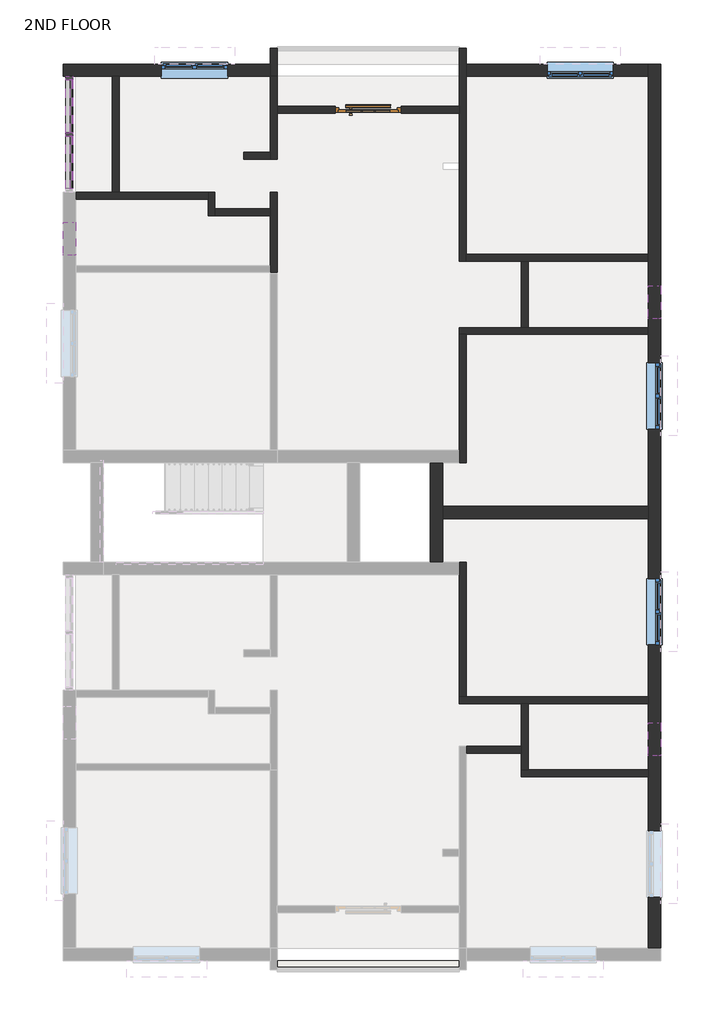
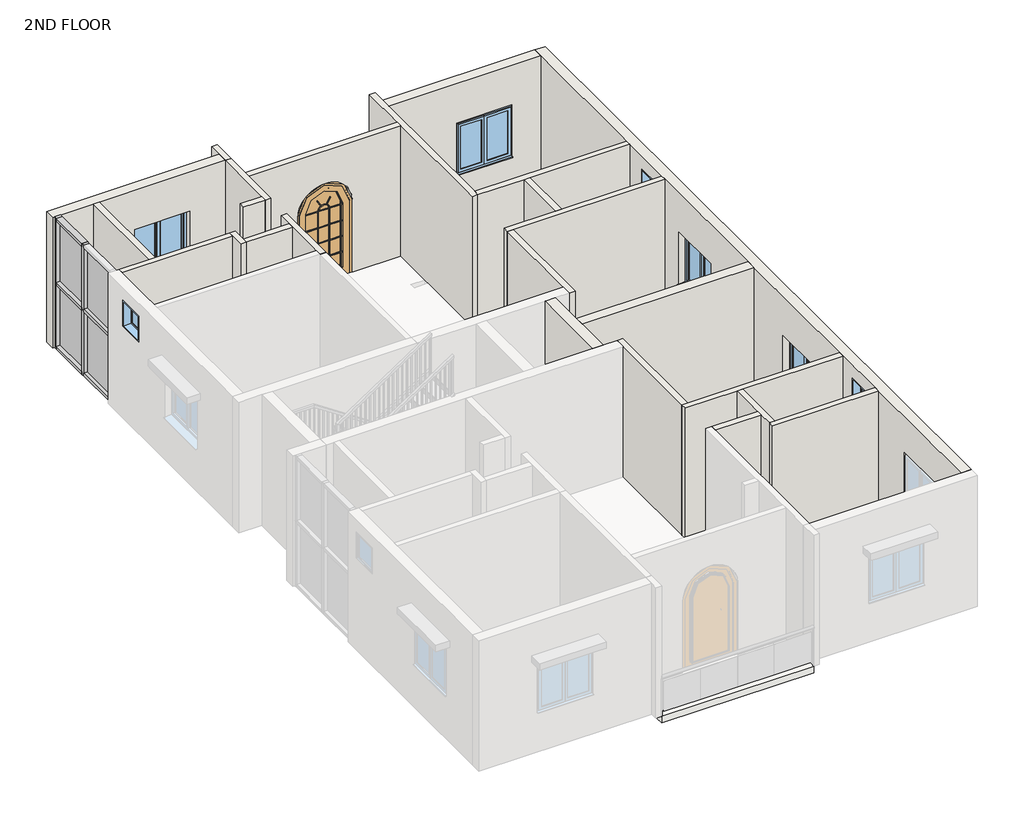
# One storey, part 2 of 4: 24 walls, 9 members, 7 windows, 4 plates, 1 door, 1 slab.
"""IFC4 building model written with IfcOpenShell, lengths in millimetres."""

from ifc_helpers import new_model, si_unit, point, frame, frame_2d, origin, place, context, project, spatial, polyline, circle_curve, trimmed, segment, composite_curve, outline, extrude, faceted_brep, transform, mapped, element, save
from components import door_arched_single_french_glass_wood_exterior_4_x_7_french_5c4dec95, member_801a2072, member_82905deb, member_88aa5c81, member_4491d118, system_panel_glazed_a8655be6, window_80340324, w2_windows_4_x_4_9dec5fc7

model = new_model("IFC4")

# Units and contexts
model_context = context("Model", 3, world=origin())
ifc_project = project(units=[si_unit("LENGTHUNIT", "METRE", prefix="MILLI")], contexts=[model_context])

# Site, building, storey
site = spatial("IfcSite", under=ifc_project)
building = spatial("IfcBuilding", under=site)
storey = spatial("IfcBuildingStorey", under=building, Name="2ND FLOOR", Elevation=9144.0)

# Door
placement = place(None, origin())
door_arched_single_french_glass_wood_exterior_4_x_7_french_shape = door_arched_single_french_glass_wood_exterior_4_x_7_french_5c4dec95(model_context)
element("IfcDoor", 1, ObjectType="Door_Arched_Single_French_Glass_Wood_Exterior : 4' x 7' french door", at=placement, inside=storey, context=model_context, shape_type="MappedRepresentation", body=[
    mapped(door_arched_single_french_glass_wood_exterior_4_x_7_french_shape, transform((-817.6012202, 12433.0309003, 9144.0), x_axis=(1.0, 0.0, 0.0), y_axis=(0.0, 1.0, 0.0), z_axis=(0.0, 0.0, 1.0))),
])

# Members
member_shape = member_801a2072(model_context)
element("IfcMember", 2, ObjectType="Rectangular Mullion : 2.5\" x 5\" rectangular", at=placement, inside=storey, context=model_context, shape_type="MappedRepresentation", body=[
    mapped(member_shape, transform((-6318.2887202, 12007.5809003, 12192.0), x_axis=(0.0, 0.0, 1.0), y_axis=(-1.0, 0.0, 0.0), z_axis=(0.0, -1.0, 0.0))),
])
element("IfcMember", 3, ObjectType="Rectangular Mullion : 2.5\" x 5\" rectangular", at=placement, inside=storey, context=model_context, shape_type="MappedRepresentation", body=[
    mapped(member_shape, transform((-6318.2887202, 12979.1309003, 9144.0), x_axis=(0.0, 0.0, -1.0), y_axis=(-1.0, 0.0, 0.0), z_axis=(0.0, 1.0, 0.0))),
])
element("IfcMember", 4, ObjectType="Rectangular Mullion : 2.5\" x 5\" rectangular", at=placement, inside=storey, context=model_context, shape_type="MappedRepresentation", body=[
    mapped(member_shape, transform((-6318.2887202, 11944.0809003, 9144.0), x_axis=(0.0, 0.0, -1.0), y_axis=(-1.0, 0.0, 0.0), z_axis=(0.0, 1.0, 0.0))),
])
member_2_shape = member_82905deb(model_context)
element("IfcMember", 5, ObjectType="Rectangular Mullion : 2.5\" x 5\" rectangular", at=placement, inside=storey, context=model_context, shape_type="MappedRepresentation", body=[
    mapped(member_2_shape, transform((-6318.2887202, 11975.8309003, 9144.0), x_axis=(0.0, -1.0, 0.0), y_axis=(-1.0, 0.0, 0.0), z_axis=(0.0, 0.0, -1.0))),
])
member_3_shape = member_88aa5c81(model_context)
element("IfcMember", 6, ObjectType="Rectangular Mullion : 2.5\" x 5\" rectangular", at=placement, inside=storey, context=model_context, shape_type="MappedRepresentation", body=[
    mapped(member_3_shape, transform((-6318.2887202, 12007.5809003, 10668.0), x_axis=(0.0, 0.0, 1.0), y_axis=(-1.0, 0.0, 0.0), z_axis=(0.0, -1.0, 0.0))),
])
element("IfcMember", 7, ObjectType="Rectangular Mullion : 2.5\" x 5\" rectangular", at=placement, inside=storey, context=model_context, shape_type="MappedRepresentation", body=[
    mapped(member_3_shape, transform((-6318.2887202, 10972.5309003, 10668.0), x_axis=(0.0, 0.0, 1.0), y_axis=(-1.0, 0.0, 0.0), z_axis=(0.0, -1.0, 0.0))),
])
element("IfcMember", 8, ObjectType="Rectangular Mullion : 2.5\" x 5\" rectangular", at=placement, inside=storey, context=model_context, shape_type="MappedRepresentation", body=[
    mapped(member_2_shape, transform((-6318.2887202, 11975.8309003, 10668.0), x_axis=(0.0, -1.0, 0.0), y_axis=(-1.0, 0.0, 0.0), z_axis=(0.0, 0.0, -1.0))),
])
member_4_shape = member_4491d118(model_context)
element("IfcMember", 9, ObjectType="Rectangular Mullion : 2.5\" x 5\" rectangular", at=placement, inside=storey, context=model_context, shape_type="MappedRepresentation", body=[
    mapped(member_4_shape, transform((-6318.2887202, 13042.6309003, 12192.0), x_axis=(0.0, 1.0, 0.0), y_axis=(-1.0, 0.0, 0.0), z_axis=(0.0, 0.0, 1.0))),
])
element("IfcMember", 10, ObjectType="Rectangular Mullion : 2.5\" x 5\" rectangular", at=placement, inside=storey, context=model_context, shape_type="MappedRepresentation", body=[
    mapped(member_4_shape, transform((-6318.2887202, 13042.6309003, 10668.0), x_axis=(0.0, 1.0, 0.0), y_axis=(-1.0, 0.0, 0.0), z_axis=(0.0, 0.0, 1.0))),
])

# Plates
system_panel_glazed_shape = system_panel_glazed_a8655be6(model_context)
element("IfcPlate", 11, ObjectType="System Panel : Glazed", at=placement, inside=storey, context=model_context, shape_type="MappedRepresentation", body=[
    mapped(system_panel_glazed_shape, transform((-6318.2887202, 12493.3559003, 9207.5), x_axis=(0.0, -1.0, 0.0), y_axis=(1.0, 0.0, 0.0), z_axis=(0.0, 0.0, 1.0))),
])
element("IfcPlate", 12, ObjectType="System Panel : Glazed", at=placement, inside=storey, context=model_context, shape_type="MappedRepresentation", body=[
    mapped(system_panel_glazed_shape, transform((-6318.2887202, 11458.3059003, 9207.5), x_axis=(0.0, -1.0, 0.0), y_axis=(1.0, 0.0, 0.0), z_axis=(0.0, 0.0, 1.0))),
])
element("IfcPlate", 13, ObjectType="System Panel : Glazed", at=placement, inside=storey, context=model_context, shape_type="MappedRepresentation", body=[
    mapped(system_panel_glazed_shape, transform((-6318.2887202, 12493.3559003, 10699.75), x_axis=(0.0, -1.0, 0.0), y_axis=(1.0, 0.0, 0.0), z_axis=(0.0, 0.0, 1.0))),
])
element("IfcPlate", 14, ObjectType="System Panel : Glazed", at=placement, inside=storey, context=model_context, shape_type="MappedRepresentation", body=[
    mapped(system_panel_glazed_shape, transform((-6318.2887202, 11458.3059003, 10699.75), x_axis=(0.0, -1.0, 0.0), y_axis=(1.0, 0.0, 0.0), z_axis=(0.0, 0.0, 1.0))),
])

# Slab
element("IfcSlab", 15, ObjectType="bathroom tiles", at=placement, inside=storey, context=model_context, shape_type="SweptSolid", body=[
    extrude(outline(polyline([(858.7987798, -3238.7690997), (858.7987798, -3403.8690997), (-2494.0012202, -3403.8690997), (-2494.0012202, -3238.7690997), (858.7987798, -3238.7690997)])), frame((0.0, 0.0, 8991.6), z_axis=(0.0, 0.0, 1.0), x_axis=(1.0, 0.0, 0.0)), (0.0, 0.0, 1.0), 152.4),
])

# Walls
element("IfcWall", 16, ObjectType="OUTER WALL 9\"", at=placement, inside=storey, context=model_context, shape_type="Brep", body=[
    faceted_brep([(4567.1987798, -3010.1690997, 9144.0), (4567.1987798, 13271.2309003, 9144.0), (4567.1987798, 13271.2309003, 12192.0), (4567.1987798, -3010.1690997, 12192.0), (4567.1987798, -844.8190997, 11363.2), (4567.1987798, -844.8190997, 10144.0), (4567.1987798, -2064.0190997, 10144.0), (4567.1987798, -2064.0190997, 11363.2), (4567.1987798, 2577.8309003, 10058.4), (4567.1987798, 2577.8309003, 11277.6), (4567.1987798, 3797.0309003, 11277.6), (4567.1987798, 3797.0309003, 10058.4), (4567.1987798, 6552.9309003, 10058.4), (4567.1987798, 6552.9309003, 11277.6), (4567.1987798, 7772.1309003, 11277.6), (4567.1987798, 7772.1309003, 10058.4), (4567.1987798, 539.4809003, 11277.6), (4567.1987798, 539.4809003, 11887.2), (4567.1987798, 1149.0809003, 11887.2), (4567.1987798, 1149.0809003, 11277.6), (4567.1987798, 8584.9309003, 11277.6), (4567.1987798, 8584.9309003, 11887.2), (4567.1987798, 9194.5309003, 11887.2), (4567.1987798, 9194.5309003, 11277.6), (4338.5987798, 13271.2309003, 9144.0), (4338.5987798, 13042.6309003, 9144.0), (4338.5987798, 9766.0309003, 9144.0), (4338.5987798, 9639.0309003, 9144.0), (4338.5987798, 8419.8309003, 9144.0), (4338.5987798, 8292.8309003, 9144.0), (4338.5987798, 5130.5309003, 9144.0), (4338.5987798, 4901.9309003, 9144.0), (4338.5987798, 1625.3309003, 9144.0), (4338.5987798, 1498.3309003, 9144.0), (4338.5987798, 279.1309003, 9144.0), (4338.5987798, 152.1309003, 9144.0), (4338.5987798, -3010.1690997, 9144.0), (4338.5987798, -3010.1690997, 12192.0), (4338.5987798, 152.1309003, 12192.0), (4338.5987798, 279.1309003, 12192.0), (4338.5987798, 1498.3309003, 12192.0), (4338.5987798, 1625.3309003, 12192.0), (4338.5987798, 4901.9309003, 12192.0), (4338.5987798, 5130.5309003, 12192.0), (4338.5987798, 8292.8309003, 12192.0), (4338.5987798, 8419.8309003, 12192.0), (4338.5987798, 9639.0309003, 12192.0), (4338.5987798, 9766.0309003, 12192.0), (4338.5987798, 13042.6309003, 12192.0), (4338.5987798, 13271.2309003, 12192.0), (4338.5987798, -844.8190997, 10144.0), (4338.5987798, -844.8190997, 11363.2), (4338.5987798, -2064.0190997, 11363.2), (4338.5987798, -2064.0190997, 10144.0), (4338.5987798, 2577.8309003, 11277.6), (4338.5987798, 2577.8309003, 10058.4), (4338.5987798, 3797.0309003, 10058.4), (4338.5987798, 3797.0309003, 11277.6), (4338.5987798, 6552.9309003, 11277.6), (4338.5987798, 6552.9309003, 10058.4), (4338.5987798, 7772.1309003, 10058.4), (4338.5987798, 7772.1309003, 11277.6), (4338.5987798, 539.4809003, 11887.2), (4338.5987798, 539.4809003, 11277.6), (4338.5987798, 1149.0809003, 11277.6), (4338.5987798, 1149.0809003, 11887.2), (4338.5987798, 8584.9309003, 11887.2), (4338.5987798, 8584.9309003, 11277.6), (4338.5987798, 9194.5309003, 11277.6), (4338.5987798, 9194.5309003, 11887.2)], [[[0, 1, 2, 3], [4, 5, 6, 7], [8, 9, 10, 11], [12, 13, 14, 15], [16, 17, 18, 19], [20, 21, 22, 23]], [[24, 25, 26, 27, 28, 29, 30, 31, 32, 33, 34, 35, 36, 37, 38, 39, 40, 41, 42, 43, 44, 45, 46, 47, 48, 49], [50, 51, 52, 53], [54, 55, 56, 57], [58, 59, 60, 61], [62, 63, 64, 65], [66, 67, 68, 69]], [[1, 0, 36, 35, 34, 33, 32, 31, 30, 29, 28, 27, 26, 25, 24]], [[3, 2, 49, 48, 47, 46, 45, 44, 43, 42, 41, 40, 39, 38, 37]], [[0, 3, 37, 36]], [[2, 1, 24, 49]], [[51, 50, 5, 4]], [[52, 51, 4, 7]], [[53, 52, 7, 6]], [[50, 53, 6, 5]], [[9, 8, 55, 54]], [[10, 9, 54, 57]], [[11, 10, 57, 56]], [[8, 11, 56, 55]], [[13, 12, 59, 58]], [[14, 13, 58, 61]], [[15, 14, 61, 60]], [[12, 15, 60, 59]], [[63, 62, 17, 16]], [[64, 63, 16, 19]], [[65, 64, 19, 18]], [[62, 65, 18, 17]], [[67, 66, 21, 20]], [[68, 67, 20, 23]], [[69, 68, 23, 22]], [[66, 69, 22, 21]]]),
])
element("IfcWall", 17, ObjectType="OUTER WALL 9\"", at=placement, inside=storey, context=model_context, shape_type="SweptSolid", body=[
    extrude(outline(polyline([(9144.0, 4338.5987798), (12192.0, 4338.5987798), (12192.0, 985.7987798), (9144.0, 985.7987798), (9144.0, 4338.5987798)]), holes=[polyline([(10058.4, 2479.7847416), (11277.6, 2479.7847416), (11277.6, 3698.9847416), (10058.4, 3698.9847416), (10058.4, 2479.7847416)])]), frame((0.0, 13042.6309003, 0.0), z_axis=(0.0, 1.0, 0.0), x_axis=(0.0, 0.0, 1.0)), (0.0, 0.0, 1.0), 228.6),
])
element("IfcWall", 18, ObjectType="OUTER WALL 9\"", at=placement, inside=storey, context=model_context, shape_type="Brep", body=[
    faceted_brep([(-2621.0012202, 13271.2309003, 9144.0), (-6432.5887202, 13271.2309003, 9144.0), (-6432.5887202, 13271.2309003, 12192.0), (-2621.0012202, 13271.2309003, 12192.0), (-3402.0512202, 13271.2309003, 10058.4), (-3402.0512202, 13271.2309003, 11277.6), (-4621.2512202, 13271.2309003, 11277.6), (-4621.2512202, 13271.2309003, 10058.4), (-2621.0012202, 13042.6309003, 9144.0), (-2621.0012202, 13042.6309003, 12192.0), (-5402.3012202, 13042.6309003, 12192.0), (-5529.3012202, 13042.6309003, 12192.0), (-6432.5887202, 13042.6309003, 12192.0), (-6432.5887202, 13042.6309003, 9144.0), (-5529.3012202, 13042.6309003, 9144.0), (-5402.3012202, 13042.6309003, 9144.0), (-3402.0512202, 13042.6309003, 10058.4), (-4621.2512202, 13042.6309003, 10058.4), (-4621.2512202, 13042.6309003, 11277.6), (-3402.0512202, 13042.6309003, 11277.6)], [[[0, 1, 2, 3], [4, 5, 6, 7]], [[8, 9, 10, 11, 12, 13, 14, 15], [16, 17, 18, 19]], [[1, 0, 8, 15, 14, 13]], [[3, 2, 12, 11, 10, 9]], [[2, 1, 13, 12]], [[5, 4, 16, 19]], [[6, 5, 19, 18]], [[7, 6, 18, 17]], [[4, 7, 17, 16]], [[0, 3, 9, 8]]]),
])
element("IfcWall", 19, ObjectType="OUTER WALL 9\"", at=placement, inside=storey, context=model_context, shape_type="Brep", body=[
    faceted_brep([(553.9987798, 4101.8309003, 9144.0), (553.9987798, 4901.9309003, 9144.0), (553.9987798, 5130.5309003, 9144.0), (553.9987798, 5930.6309003, 9144.0), (553.9987798, 5930.6309003, 12192.0), (553.9987798, 5130.5309003, 12192.0), (553.9987798, 4901.9309003, 12192.0), (553.9987798, 4101.8309003, 12192.0), (325.3987798, 4101.8309003, 9144.0), (325.3987798, 4101.8309003, 12192.0), (325.3987798, 5930.6309003, 12192.0), (325.3987798, 5930.6309003, 9144.0)], [[[0, 1, 2, 3, 4, 5, 6, 7]], [[8, 9, 10, 11]], [[3, 2, 1, 0, 8, 11]], [[7, 6, 5, 4, 10, 9]], [[0, 7, 9, 8]], [[4, 3, 11, 10]]]),
])
element("IfcWall", 20, ObjectType="OUTER WALL 9\"", at=placement, inside=storey, context=model_context, shape_type="SweptSolid", body=[
    extrude(outline(polyline([(4338.5987798, 4901.9309003), (553.9987798, 4901.9309003), (553.9987798, 5130.5309003), (4338.5987798, 5130.5309003), (4338.5987798, 4901.9309003)])), frame((0.0, 0.0, 9144.0), z_axis=(0.0, 0.0, 1.0), x_axis=(1.0, 0.0, 0.0)), (0.0, 0.0, 1.0), 3048.0),
])
element("IfcWall", 21, ObjectType="inner wall 5\"", at=placement, inside=storey, context=model_context, shape_type="SweptSolid", body=[
    extrude(outline(polyline([(-5529.3012202, 10909.0309003), (-5529.3012202, 13042.6309003), (-5402.3012202, 13042.6309003), (-5402.3012202, 10909.0309003), (-5529.3012202, 10909.0309003)])), frame((0.0, 0.0, 9144.0), z_axis=(0.0, 0.0, 1.0), x_axis=(1.0, 0.0, 0.0)), (0.0, 0.0, 1.0), 3048.0),
])
element("IfcWall", 22, ObjectType="inner wall 5\"", at=placement, inside=storey, context=model_context, shape_type="Brep", body=[
    faceted_brep([(-2621.0012202, 13042.6309003, 9144.0), (-2621.0012202, 11645.6309003, 9144.0), (-2621.0012202, 11518.6309003, 9144.0), (-2621.0012202, 11518.6309003, 12192.0), (-2621.0012202, 11645.6309003, 12192.0), (-2621.0012202, 13042.6309003, 12192.0), (-2494.0012202, 13042.6309003, 9144.0), (-2494.0012202, 13042.6309003, 12192.0), (-2494.0012202, 12496.5309003, 12192.0), (-2494.0012202, 12369.5309003, 12192.0), (-2494.0012202, 11518.6309003, 12192.0), (-2494.0012202, 11518.6309003, 9144.0), (-2494.0012202, 12369.5309003, 9144.0), (-2494.0012202, 12496.5309003, 9144.0)], [[[0, 1, 2, 3, 4, 5]], [[6, 7, 8, 9, 10, 11, 12, 13]], [[2, 1, 0, 6, 13, 12, 11]], [[5, 4, 3, 10, 9, 8, 7]], [[3, 2, 11, 10]], [[0, 5, 7, 6]]]),
])
element("IfcWall", 23, ObjectType="inner wall 5\"", at=placement, inside=storey, context=model_context, shape_type="SweptSolid", body=[
    extrude(outline(polyline([(-3103.6012202, 11645.6309003), (-2621.0012202, 11645.6309003), (-2621.0012202, 11518.6309003), (-3103.6012202, 11518.6309003), (-3103.6012202, 11645.6309003)])), frame((0.0, 0.0, 9144.0), z_axis=(0.0, 0.0, 1.0), x_axis=(1.0, 0.0, 0.0)), (0.0, 0.0, 1.0), 3048.0),
])
element("IfcWall", 24, ObjectType="inner wall 5\"", at=placement, inside=storey, context=model_context, shape_type="Brep", body=[
    faceted_brep([(-6202.4012202, 10782.0309003, 9144.0), (-3764.0012202, 10782.0309003, 9144.0), (-3764.0012202, 10782.0309003, 12192.0), (-6202.4012202, 10782.0309003, 12192.0), (-6202.4012202, 10909.0309003, 9144.0), (-6202.4012202, 10909.0309003, 12192.0), (-5529.3012202, 10909.0309003, 12192.0), (-5402.3012202, 10909.0309003, 12192.0), (-3764.0012202, 10909.0309003, 12192.0), (-3764.0012202, 10909.0309003, 9144.0), (-5402.3012202, 10909.0309003, 9144.0), (-5529.3012202, 10909.0309003, 9144.0)], [[[0, 1, 2, 3]], [[4, 5, 6, 7, 8, 9, 10, 11]], [[1, 0, 4, 11, 10, 9]], [[3, 2, 8, 7, 6, 5]], [[0, 3, 5, 4]], [[2, 1, 9, 8]]]),
])
element("IfcWall", 25, ObjectType="inner wall 5\"", at=placement, inside=storey, context=model_context, shape_type="Brep", body=[
    faceted_brep([(-3764.0012202, 10909.0309003, 9144.0), (-3764.0012202, 10782.0309003, 9144.0), (-3764.0012202, 10477.2309003, 9144.0), (-3764.0012202, 10477.2309003, 12192.0), (-3764.0012202, 10782.0309003, 12192.0), (-3764.0012202, 10909.0309003, 12192.0), (-3637.0012202, 10909.0309003, 9144.0), (-3637.0012202, 10909.0309003, 12192.0), (-3637.0012202, 10604.2309003, 12192.0), (-3637.0012202, 10477.2309003, 12192.0), (-3637.0012202, 10477.2309003, 9144.0), (-3637.0012202, 10604.2309003, 9144.0)], [[[0, 1, 2, 3, 4, 5]], [[6, 7, 8, 9, 10, 11]], [[2, 1, 0, 6, 11, 10]], [[5, 4, 3, 9, 8, 7]], [[0, 5, 7, 6]], [[3, 2, 10, 9]]]),
])
element("IfcWall", 26, ObjectType="inner wall 5\"", at=placement, inside=storey, context=model_context, shape_type="SweptSolid", body=[
    extrude(outline(polyline([(-2621.0012202, 10477.2309003), (-3637.0012202, 10477.2309003), (-3637.0012202, 10604.2309003), (-2621.0012202, 10604.2309003), (-2621.0012202, 10477.2309003)])), frame((0.0, 0.0, 9144.0), z_axis=(0.0, 0.0, 1.0), x_axis=(1.0, 0.0, 0.0)), (0.0, 0.0, 1.0), 3048.0),
])
element("IfcWall", 27, ObjectType="inner wall 5\"", at=placement, inside=storey, context=model_context, shape_type="Brep", body=[
    faceted_brep([(-2621.0012202, 10909.0309003, 9144.0), (-2621.0012202, 10604.2309003, 9144.0), (-2621.0012202, 10477.2309003, 9144.0), (-2621.0012202, 9562.8309003, 9144.0), (-2621.0012202, 9435.8309003, 9144.0), (-2621.0012202, 9435.8309003, 12192.0), (-2621.0012202, 9562.8309003, 12192.0), (-2621.0012202, 10477.2309003, 12192.0), (-2621.0012202, 10604.2309003, 12192.0), (-2621.0012202, 10909.0309003, 12192.0), (-2494.0012202, 10909.0309003, 9144.0), (-2494.0012202, 10909.0309003, 12192.0), (-2494.0012202, 9435.8309003, 12192.0), (-2494.0012202, 9435.8309003, 9144.0)], [[[0, 1, 2, 3, 4, 5, 6, 7, 8, 9]], [[10, 11, 12, 13]], [[4, 3, 2, 1, 0, 10, 13]], [[9, 8, 7, 6, 5, 12, 11]], [[0, 9, 11, 10]], [[5, 4, 13, 12]]]),
])
element("IfcWall", 28, ObjectType="inner wall 5\"", at=placement, inside=storey, context=model_context, shape_type="SweptSolid", body=[
    extrude(outline(polyline([(2001.7987798, 583.9309003), (985.7987798, 583.9309003), (985.7987798, 710.9309003), (2001.7987798, 710.9309003), (2001.7987798, 583.9309003)])), frame((0.0, 0.0, 9144.0), z_axis=(0.0, 0.0, 1.0), x_axis=(1.0, 0.0, 0.0)), (0.0, 0.0, 1.0), 3048.0),
])
element("IfcWall", 29, ObjectType="inner wall 5\"", at=placement, inside=storey, context=model_context, shape_type="Brep", body=[
    faceted_brep([(4338.5987798, 1625.3309003, 9144.0), (985.7987798, 1625.3309003, 9144.0), (858.7987798, 1625.3309003, 9144.0), (858.7987798, 1625.3309003, 12192.0), (985.7987798, 1625.3309003, 12192.0), (4338.5987798, 1625.3309003, 12192.0), (4338.5987798, 1498.3309003, 9144.0), (4338.5987798, 1498.3309003, 12192.0), (2128.7987798, 1498.3309003, 12192.0), (2001.7987798, 1498.3309003, 12192.0), (858.7987798, 1498.3309003, 12192.0), (858.7987798, 1498.3309003, 9144.0), (2001.7987798, 1498.3309003, 9144.0), (2128.7987798, 1498.3309003, 9144.0)], [[[0, 1, 2, 3, 4, 5]], [[6, 7, 8, 9, 10, 11, 12, 13]], [[2, 1, 0, 6, 13, 12, 11]], [[5, 4, 3, 10, 9, 8, 7]], [[3, 2, 11, 10]], [[0, 5, 7, 6]]]),
])
element("IfcWall", 30, ObjectType="inner wall 5\"", at=placement, inside=storey, context=model_context, shape_type="Brep", body=[
    faceted_brep([(985.7987798, 1625.3309003, 9144.0), (985.7987798, 4101.8309003, 9144.0), (985.7987798, 4101.8309003, 12192.0), (985.7987798, 1625.3309003, 12192.0), (858.7987798, 1625.3309003, 9144.0), (858.7987798, 1625.3309003, 12192.0), (858.7987798, 3873.2309003, 12192.0), (858.7987798, 4101.8309003, 12192.0), (858.7987798, 4101.8309003, 9144.0), (858.7987798, 3873.2309003, 9144.0)], [[[0, 1, 2, 3]], [[4, 5, 6, 7, 8, 9]], [[1, 0, 4, 9, 8]], [[3, 2, 7, 6, 5]], [[0, 3, 5, 4]], [[2, 1, 8, 7]]]),
])
element("IfcWall", 31, ObjectType="inner wall 5\"", at=placement, inside=storey, context=model_context, shape_type="Brep", body=[
    faceted_brep([(4338.5987798, 279.1309003, 9144.0), (2128.7987798, 279.1309003, 9144.0), (2001.7987798, 279.1309003, 9144.0), (2001.7987798, 279.1309003, 12192.0), (2128.7987798, 279.1309003, 12192.0), (4338.5987798, 279.1309003, 12192.0), (4338.5987798, 152.1309003, 9144.0), (4338.5987798, 152.1309003, 12192.0), (2001.7987798, 152.1309003, 12192.0), (2001.7987798, 152.1309003, 9144.0)], [[[0, 1, 2, 3, 4, 5]], [[6, 7, 8, 9]], [[2, 1, 0, 6, 9]], [[5, 4, 3, 8, 7]], [[0, 5, 7, 6]], [[3, 2, 9, 8]]]),
])
element("IfcWall", 32, ObjectType="inner wall 5\"", at=placement, inside=storey, context=model_context, shape_type="Brep", body=[
    faceted_brep([(2128.7987798, 279.1309003, 9144.0), (2128.7987798, 1498.3309003, 9144.0), (2128.7987798, 1498.3309003, 12192.0), (2128.7987798, 279.1309003, 12192.0), (2001.7987798, 279.1309003, 9144.0), (2001.7987798, 279.1309003, 12192.0), (2001.7987798, 583.9309003, 12192.0), (2001.7987798, 710.9309003, 12192.0), (2001.7987798, 1498.3309003, 12192.0), (2001.7987798, 1498.3309003, 9144.0), (2001.7987798, 710.9309003, 9144.0), (2001.7987798, 583.9309003, 9144.0)], [[[0, 1, 2, 3]], [[4, 5, 6, 7, 8, 9, 10, 11]], [[1, 0, 4, 11, 10, 9]], [[3, 2, 8, 7, 6, 5]], [[0, 3, 5, 4]], [[2, 1, 9, 8]]]),
])
element("IfcWall", 33, ObjectType="inner wall 5\"", at=placement, inside=storey, context=model_context, shape_type="SweptSolid", body=[
    extrude(outline(composite_curve([segment(polyline([(10822.6, -208.0012202), (9144.0, -208.0012202), (9144.0, 858.7987798), (12192.0, 858.7987798), (12192.0, -2494.0012202), (9144.0, -2494.0012202), (9144.0, -1427.2012202), (10822.6, -1427.2012202)]), True, "CONTINUOUS"), segment(trimmed(circle_curve(frame_2d((10822.6, -817.6012202)), 609.6), [point((10822.6, -1427.2012202))], [point((10822.6, -208.0012202))], True, "CARTESIAN"), True, "CONTINUOUS")], self_intersect=False)), frame((0.0, 12369.5309003, 0.0), z_axis=(0.0, 1.0, 0.0), x_axis=(0.0, 0.0, 1.0)), (0.0, 0.0, 1.0), 127.0),
])
element("IfcWall", 34, ObjectType="inner wall 5\"", at=placement, inside=storey, context=model_context, shape_type="Brep", body=[
    faceted_brep([(858.7987798, 13563.3309003, 9144.0), (858.7987798, 12496.5309003, 9144.0), (858.7987798, 12369.5309003, 9144.0), (858.7987798, 9639.0309003, 9144.0), (858.7987798, 9639.0309003, 12192.0), (858.7987798, 12369.5309003, 12192.0), (858.7987798, 12496.5309003, 12192.0), (858.7987798, 13563.3309003, 12192.0), (985.7987798, 13563.3309003, 9144.0), (985.7987798, 13563.3309003, 12192.0), (985.7987798, 13271.2309003, 12192.0), (985.7987798, 13042.6309003, 12192.0), (985.7987798, 9766.0309003, 12192.0), (985.7987798, 9639.0309003, 12192.0), (985.7987798, 9639.0309003, 9144.0), (985.7987798, 9766.0309003, 9144.0), (985.7987798, 13042.6309003, 9144.0), (985.7987798, 13271.2309003, 9144.0)], [[[0, 1, 2, 3, 4, 5, 6, 7]], [[8, 9, 10, 11, 12, 13, 14, 15, 16, 17]], [[3, 2, 1, 0, 8, 17, 16, 15, 14]], [[7, 6, 5, 4, 13, 12, 11, 10, 9]], [[0, 7, 9, 8]], [[4, 3, 14, 13]]]),
])
element("IfcWall", 35, ObjectType="inner wall 5\"", at=placement, inside=storey, context=model_context, shape_type="Brep", body=[
    faceted_brep([(4338.5987798, 9766.0309003, 9144.0), (985.7987798, 9766.0309003, 9144.0), (985.7987798, 9766.0309003, 12192.0), (4338.5987798, 9766.0309003, 12192.0), (4338.5987798, 9639.0309003, 9144.0), (4338.5987798, 9639.0309003, 12192.0), (2128.7987798, 9639.0309003, 12192.0), (2001.7987798, 9639.0309003, 12192.0), (985.7987798, 9639.0309003, 12192.0), (985.7987798, 9639.0309003, 9144.0), (2001.7987798, 9639.0309003, 9144.0), (2128.7987798, 9639.0309003, 9144.0)], [[[0, 1, 2, 3]], [[4, 5, 6, 7, 8, 9, 10, 11]], [[1, 0, 4, 11, 10, 9]], [[3, 2, 8, 7, 6, 5]], [[0, 3, 5, 4]], [[2, 1, 9, 8]]]),
])
element("IfcWall", 36, ObjectType="inner wall 5\"", at=placement, inside=storey, context=model_context, shape_type="Brep", body=[
    faceted_brep([(4338.5987798, 8419.8309003, 9144.0), (2128.7987798, 8419.8309003, 9144.0), (2001.7987798, 8419.8309003, 9144.0), (858.7987798, 8419.8309003, 9144.0), (858.7987798, 8419.8309003, 12192.0), (2001.7987798, 8419.8309003, 12192.0), (2128.7987798, 8419.8309003, 12192.0), (4338.5987798, 8419.8309003, 12192.0), (4338.5987798, 8292.8309003, 9144.0), (4338.5987798, 8292.8309003, 12192.0), (985.7987798, 8292.8309003, 12192.0), (858.7987798, 8292.8309003, 12192.0), (858.7987798, 8292.8309003, 9144.0), (985.7987798, 8292.8309003, 9144.0)], [[[0, 1, 2, 3, 4, 5, 6, 7]], [[8, 9, 10, 11, 12, 13]], [[3, 2, 1, 0, 8, 13, 12]], [[7, 6, 5, 4, 11, 10, 9]], [[0, 7, 9, 8]], [[4, 3, 12, 11]]]),
])
element("IfcWall", 37, ObjectType="inner wall 5\"", at=placement, inside=storey, context=model_context, shape_type="SweptSolid", body=[
    extrude(outline(polyline([(2128.7987798, 9639.0309003), (2128.7987798, 8419.8309003), (2001.7987798, 8419.8309003), (2001.7987798, 9639.0309003), (2128.7987798, 9639.0309003)])), frame((0.0, 0.0, 9144.0), z_axis=(0.0, 0.0, 1.0), x_axis=(1.0, 0.0, 0.0)), (0.0, 0.0, 1.0), 3048.0),
])
element("IfcWall", 38, ObjectType="inner wall 5\"", at=placement, inside=storey, context=model_context, shape_type="Brep", body=[
    faceted_brep([(858.7987798, 8292.8309003, 9144.0), (858.7987798, 6159.2309003, 9144.0), (858.7987798, 5930.6309003, 9144.0), (858.7987798, 5930.6309003, 12192.0), (858.7987798, 6159.2309003, 12192.0), (858.7987798, 8292.8309003, 12192.0), (985.7987798, 8292.8309003, 9144.0), (985.7987798, 8292.8309003, 12192.0), (985.7987798, 5930.6309003, 12192.0), (985.7987798, 5930.6309003, 9144.0)], [[[0, 1, 2, 3, 4, 5]], [[6, 7, 8, 9]], [[2, 1, 0, 6, 9]], [[5, 4, 3, 8, 7]], [[0, 5, 7, 6]], [[3, 2, 9, 8]]]),
])
element("IfcWall", 39, ObjectType="inner wall 5\"", at=placement, inside=storey, context=model_context, shape_type="Brep", body=[
    faceted_brep([(-2494.0012202, 13042.6309003, 9144.0), (-2494.0012202, 13563.3309003, 9144.0), (-2494.0012202, 13563.3309003, 12192.0), (-2494.0012202, 13042.6309003, 12192.0), (-2621.0012202, 13042.6309003, 9144.0), (-2621.0012202, 13042.6309003, 12192.0), (-2621.0012202, 13271.2309003, 12192.0), (-2621.0012202, 13563.3309003, 12192.0), (-2621.0012202, 13563.3309003, 9144.0), (-2621.0012202, 13271.2309003, 9144.0)], [[[0, 1, 2, 3]], [[4, 5, 6, 7, 8, 9]], [[1, 0, 4, 9, 8]], [[2, 1, 8, 7]], [[3, 2, 7, 6, 5]], [[0, 3, 5, 4]]]),
])

# Windows
window_shape = window_80340324(model_context)
element("IfcWindow", 40, ObjectType="Fixed : 24\" x 24\"", at=placement, inside=storey, context=model_context, shape_type="MappedRepresentation", body=[
    mapped(window_shape, transform((4452.8987798, 8851.6309003, 10363.2), x_axis=(0.0, -1.0, 0.0), y_axis=(1.0, 0.0, 0.0), z_axis=(0.0, 0.0, 1.0))),
])
element("IfcWindow", 41, ObjectType="Fixed : 24\" x 24\"", at=placement, inside=storey, context=model_context, shape_type="MappedRepresentation", body=[
    mapped(window_shape, transform((4452.8987798, 806.1809003, 10363.2), x_axis=(0.0, -1.0, 0.0), y_axis=(1.0, 0.0, 0.0), z_axis=(0.0, 0.0, 1.0))),
])
element("IfcWindow", 42, ObjectType="Fixed : 24\" x 24\"", at=placement, inside=storey, context=model_context, shape_type="MappedRepresentation", body=[
    mapped(window_shape, transform((-6318.2887202, 10020.0309003, 10363.2), x_axis=(0.0, -1.0, 0.0), y_axis=(1.0, 0.0, 0.0), z_axis=(0.0, 0.0, 1.0))),
])
w2_windows_4_x_4_shape = w2_windows_4_x_4_9dec5fc7(model_context)
element("IfcWindow", 43, ObjectType="w2 : windows 4' x 4'", at=placement, inside=storey, context=model_context, shape_type="MappedRepresentation", body=[
    mapped(w2_windows_4_x_4_shape, transform((3089.3847416, 13156.9309003, 9058.4), x_axis=(1.0, 0.0, 0.0), y_axis=(0.0, 1.0, 0.0), z_axis=(0.0, 0.0, 1.0))),
])
element("IfcWindow", 44, ObjectType="w2 : windows 4' x 4'", at=placement, inside=storey, context=model_context, shape_type="MappedRepresentation", body=[
    mapped(w2_windows_4_x_4_shape, transform((-4011.6512202, 13156.9309003, 9058.4), x_axis=(-1.0, 0.0, 0.0), y_axis=(0.0, -1.0, 0.0), z_axis=(0.0, 0.0, 1.0))),
])
element("IfcWindow", 45, ObjectType="w2 : windows 4' x 4'", at=placement, inside=storey, context=model_context, shape_type="MappedRepresentation", body=[
    mapped(w2_windows_4_x_4_shape, transform((4452.8987798, 7162.5309003, 9058.4), x_axis=(0.0, 1.0, 0.0), y_axis=(-1.0, 0.0, 0.0), z_axis=(0.0, 0.0, 1.0))),
])
element("IfcWindow", 46, ObjectType="w2 : windows 4' x 4'", at=placement, inside=storey, context=model_context, shape_type="MappedRepresentation", body=[
    mapped(w2_windows_4_x_4_shape, transform((4452.8987798, 3187.4309003, 9058.4), x_axis=(0.0, 1.0, 0.0), y_axis=(-1.0, 0.0, 0.0), z_axis=(0.0, 0.0, 1.0))),
])

save(model, "model.ifc")

# Revit data of these elements
# Type "Door_Arched_Single_French_Glass_Wood_Exterior : 4' x 7' french door"
#   Type Mark = "17"
#   Type Comments = "External Single"
#   Operation = "SingleSwingRight"
#   Keynote = "L20"
#   Analytic Construction = "<None>"
#   Wrap Layers (Int) from Ext = 0' - 6.98819"
#   Wrap Layers (Ext) from Ext = 0' - 4.03543"
#   Thickness = 0' - 1.73228"
#   Stile Shutting = 0' - 5.90551"
#   Stile - Top Rail = 0' - 5.90551"
#   Stile - Hanging = 0' - 5.90551"
#   Stile - Bottom Rail = 0' - 6.88976"
#   Rough Width = 4' - 0"
#   Rough Height = 7' - 0"
#   O/A Frame Width = 0' - 2.51969"
#   Handle Z Distance = 3' - 5.33858"
#   Glazing Thickness = 0' - 0.94488"
#   Glazing Bar Thickness = 0' - 0.7874"
#   FrameWidth = 0' - 1.65354"
#   FrameOffset - External = 0' - 0.98425"
#   FrameDepth = 0' - 3.50394"
#   Door Panel Width = 3' - 7.94488"
#   Handle X Distance = 0' - 2.95276"
#   Height = 7' - 0"
#   Structural Tolerance = 0' - 0.25591"
#   Tolerance = 0' - 0.11811"
#   Undercut = 0' - 0.15748"
#   Width = 4' - 0"
#   Door Panel Thickness = 0' - 1.73228"
#   Door Panel Height = 6' - 9.81496"
#   Cavity Closer Width = 0' - 1.9685"
#   Cavity Closer Offset from Ext = 0' - 4.03543"
#   Cavity Closer Depth = 0' - 3.34646"
#   Vis - Ironmongery = yes
#   Vis - Cavity Closers = yes
#   Define Thermal Properties by = 1
#   Material Glass = Door - Glazing
#   Handle Style = element 430241
#   Material Door = Door - Panel
#   Material Frame = BROWN
#   Material Ironmongery = Door - Handle
#   Function = (empty or 0)
#   Wall Closure = (empty or 0)
#   Assembly Code = ""
# Type "Rectangular Mullion : 2.5\" x 5\" rectangular"
#   built-in parameter 1007304 = 0.416667 (stored number, unit not read)
#   built-in parameter 1007301 = 0.104167 (stored number, unit not read)
#   built-in parameter 1007300 = 0.104167 (stored number, unit not read)
# Type "System Panel : Glazed"
#   Construction Type Id = "GSP4R"
#   Analytic Construction = "1/8 in Pilkington single glazing"
#   Visual Light Transmittance = 0.9
#   Solar Heat Gain Coefficient = 0.86
#   Heat Transfer Coefficient (U) = 1.18115 BTU/(h·ft²·°F)
#   Define Thermal Properties by = 1
# Type "bathroom tiles"
#   Assembly Code = "B1010"
#   Function = 0
#   Layers, outside or top first: 0' - 6" "tile flooring" (function 1)
# Type "OUTER WALL 9\""
#   Assembly Code = "B2010"
#   Layers, outside or top first: 0' - 9" "ROSE COLOUR" (function 1)
# Type "inner wall 5\""
#   Assembly Code = "B2010"
#   Layers, outside or top first: 0' - 5" "ROSE COLOUR" (function 1)
# Type "Fixed : 24\" x 24\""
#   Type Mark = "3"
#   Construction Type Id = "GSP4R"
#   Assembly Code = "B2020100"
#   Analytic Construction = "1/8 in Pilkington single glazing"
#   Visual Light Transmittance = 0.9
#   Solar Heat Gain Coefficient = 0.78
#   Heat Transfer Coefficient (U) = 0.6496 BTU/(h·ft²·°F)
#   Height = 2' - 0"
#   Default Sill Height = 3' - 0"
#   Width = 2' - 0"
#   Window Inset = 0' - 0 3/4"
#   Define Thermal Properties by = 1
#   Define Thermal Properties by = 1
#   Glass Pane Material = Glass
#   Sash Material = Sash
#   Wall Closure = (empty or 0)
# Type "w2 : windows 4' x 4'"
#   Type Mark = "31"
#   Operation = "DoublePanelVertical"
#   Keynote = "16.05.01"
#   Analytic Construction = "<None>"
#   Rough Width = 4' - 0"
#   Rough Height = 4' - 0"
#   Rahmentiefe = 0' - 2.3622"
#   Rahmenhöhe unten = 0' - 3.14961"
#   Rahmehöhe oben = 0' - 3.14961"
#   Rahmenbreite = 0' - 2.3622"
#   Heat Transfer Coefficient (U) = 2.81836 BTU/(h·ft²·°F)
#   Height = 4' - 0"
#   Flügeltiefe = 0' - 2.3622"
#   Flügelbreite = 0' - 2.3622"
#   Einbautiefe (von außen) [instance default] = 0' - 5.51181"
#   Width = 4' - 0"
#   Kippflügel [instance default] = yes
#   Drehflügel im Grundriß darstellen [instance default] = no
#   Drehflügel [instance default] = yes
#   Define Thermal Properties by = 1
#   Rahmen [instance default] = none
#   Glas [instance default] = blue glass
#   Flügel [instance default] = WINDOW COLOUR WHITE
#   Fensterbank aussen [instance default] = WINDOW COLOUR WHITE
#   Fensterbank innen [instance default] = WINDOW COLOUR WHITE
#   Visual Light Transmittance = 0
#   Thermal Resistance (R) = 0
#   Solar Heat Gain Coefficient = 0
#   Wall Closure = (empty or 0)
# Element 1 (IfcDoor, "Door_Arched_Single_French_Glass_Wood_Exterior : 4' x 7' french door")
#   Phase Created = New Construction
#   Materials on its faces: "Door - Panel", "Door - Handle", "BROWN", "Door - Glazing"
# Elements 2, 3, 4, 5, 6, 7, 8, 9, 10 (IfcMember, "Rectangular Mullion : 2.5\" x 5\" rectangular")
#   Phase Created = New Construction
#   Materials on its faces: "Aluminum"
# Elements 11, 12, 13, 14 (IfcPlate, "System Panel : Glazed")
#   Phase Created = New Construction
#   Materials on its faces: "Glass"
# Element 15 (IfcSlab, "bathroom tiles")
#   Height Offset From Level = 0' - 0"
#   Phase Created = New Construction
#   Materials on its faces: "tile flooring"
# Elements 16, 17, 18, 19, 20 (IfcWall, "OUTER WALL 9\"")
#   Top Offset = 0' - 0"
#   Base Offset = 0' - 0"
#   wall height = 10' - 0"
#   Phase Created = New Construction
#   Base Constraint = 2ND FLOOR
#   Top Constraint = 3RD FLOOR
#   Materials on its faces: "ROSE COLOUR"
# Elements 21, 22, 23, 24, 25, 26, 27, 28, 29, 30, 31, 32, 33, 34, 35, 36, 37, 38, 39 (IfcWall, "inner wall 5\"")
#   Top Offset = 0' - 0"
#   Base Offset = 0' - 0"
#   wall height = 10' - 0"
#   Phase Created = New Construction
#   Base Constraint = 2ND FLOOR
#   Top Constraint = 3RD FLOOR
#   Materials on its faces: "ROSE COLOUR"
# Element 40 (IfcWindow, "Fixed : 24\" x 24\"")
#   Mark = "46"
#   Phase Created = New Construction
#   Materials on its faces: "Sash", "Glass"
# Element 41 (IfcWindow, "Fixed : 24\" x 24\"")
#   Mark = "48"
#   Phase Created = New Construction
#   Materials on its faces: "Sash", "Glass"
# Element 42 (IfcWindow, "Fixed : 24\" x 24\"")
#   Mark = "49"
#   Phase Created = New Construction
#   Materials on its faces: "Sash", "Glass"
# Element 43 (IfcWindow, "w2 : windows 4' x 4'")
#   Mark = "37"
#   Phase Created = New Construction
#   Materials on its faces: "WINDOW COLOUR WHITE", "blue glass"
# Element 44 (IfcWindow, "w2 : windows 4' x 4'")
#   Mark = "38"
#   Phase Created = New Construction
#   Materials on its faces: "WINDOW COLOUR WHITE", "blue glass"
# Element 45 (IfcWindow, "w2 : windows 4' x 4'")
#   Mark = "41"
#   Phase Created = New Construction
#   Materials on its faces: "WINDOW COLOUR WHITE", "blue glass"
# Element 46 (IfcWindow, "w2 : windows 4' x 4'")
#   Mark = "42"
#   Phase Created = New Construction
#   Materials on its faces: "WINDOW COLOUR WHITE", "blue glass"
# Materials
#   "Door - Glazing": colour RGB 218 227 224, transparency 0.85
#   "Door - Panel": class "Wood", colour RGB 210 159 95, transparency 0, Cost = 0
#   "BROWN": class "Generic", colour RGB 120 120 120, transparency 0, Cost = 0
#   "Door - Handle": colour RGB 0 0 0, transparency 0, Keynote = "P21"
#   "tile flooring": class "Generic", colour RGB 120 120 120, transparency 0, Cost = 0
#   "ROSE COLOUR": class "Generic", colour RGB 120 120 120, transparency 0, Cost = 0
#   "Glass": class "Glass", colour RGB 0 128 192, transparency 0.75, Description = "Soda Lime Glass", Cost = 0
#   "Sash": class "Wood", colour RGB 224 178 126, transparency 0, Cost = 0
#   "blue glass": class "System", colour RGB 0 0 255, transparency 0.75, Cost = 0
#   "WINDOW COLOUR WHITE": class "Generic", colour RGB 120 120 120, transparency 0, Cost = 0
#   "Aluminum": class "Metal", colour RGB 247 247 247, transparency 0, Description = "Aluminum 6061", Cost = 0
